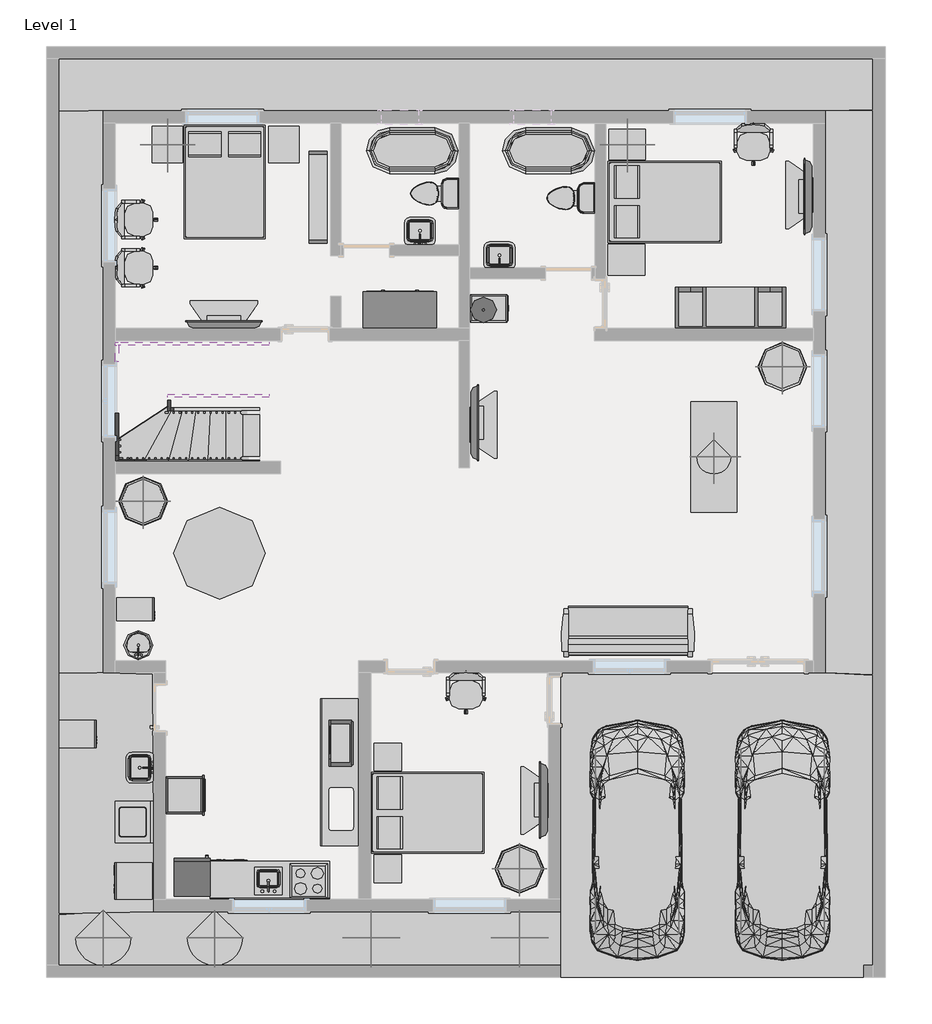
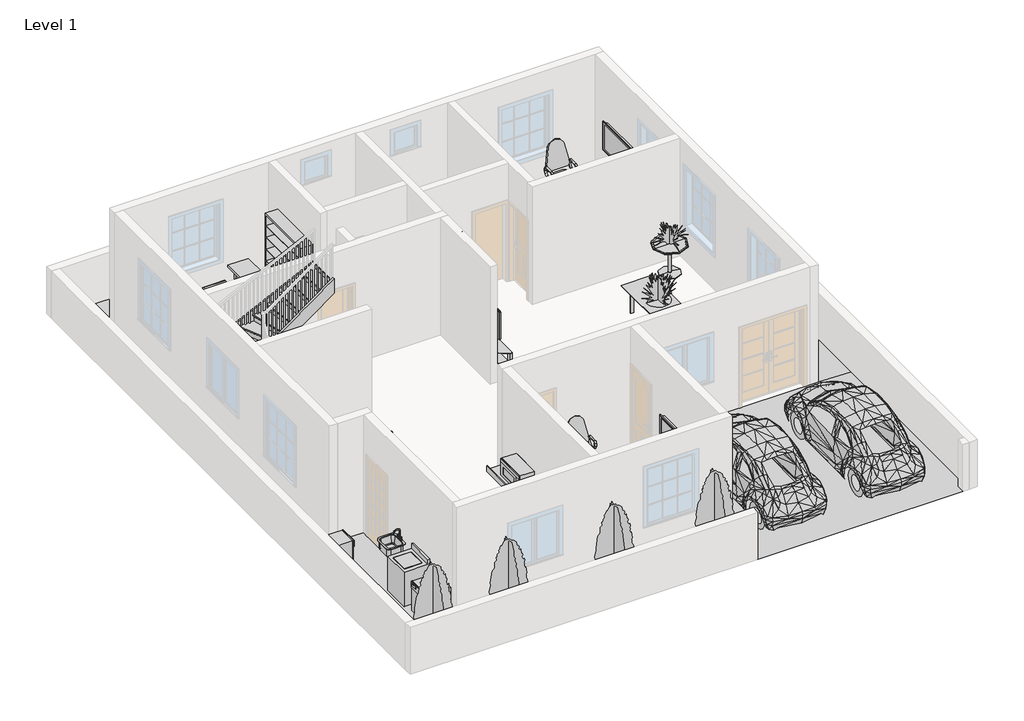
# One storey, part 3 of 3: 33 furniture elements, 18 proxies, 10 flow terminals, 10 geographic elements, 9 members, 1 stair flight.
"""IFC4 building model written with IfcOpenShell, lengths in millimetres."""

from ifc_helpers import new_model, si_unit, frame, origin, place, context, project, spatial, polyline, outline, extrude, triangles, transform, mapped, element, save
from components import proxy_db4bb64d, proxy_7e1014cc, proxy_a6faaae8, proxy_45b28599, kitchenette_medium_kitchenette_medium_844211aa, proxy_8a8d5ab2, proxy_f893816d, rpc_beetle_rpc_beetle_3ce7ba48, proxy_c523a7b7, proxy_718fa39f, flow_terminal_871c2e40, flow_terminal_d49f872f, flow_terminal_62a433f7, toilet_domestic_3d_toilet_domestic_3d_f7549cf7, toilet_domestic_3d_toilet_domestic_3d_183bbd19, flow_terminal_b374fae2, furniture_3e5ce493, furniture_c8abb964, chair_executive_chair_executive_8d69e98c, furniture_22cae41e, furniture_c6510c7c, furniture_9fa109b2, furniture_cf0b6580, furniture_b7bad97b, furniture_aff9b2fb, furniture_fdf74506, tv_stand_tv_stand_6ce107e5, furniture_c1c323c4, furniture_bbcc68ce, furniture_097b63cf, furniture_a4b90d56, furniture_eb3cba1b, rpc_plant_tropical_agave_1_5_93a2a214, rpc_plant_tropical_dagger_2_80c14bd7, rpc_tree_conifer_chinese_juniper_7_1b9786cd, stair_flight_2a3e21a6

model = new_model("IFC4")

# Units and contexts
model_context = context("Model", 3, world=origin())
ifc_project = project(units=[si_unit("LENGTHUNIT", "METRE", prefix="MILLI")], contexts=[model_context])

# Site, building, storey
site = spatial("IfcSite", under=ifc_project)
building = spatial("IfcBuilding", under=site)
storey = spatial("IfcBuildingStorey", under=building, Name="Level 1", Elevation=0.0)

# Proxies
placement = place(None, origin())
element("IfcBuildingElementProxy", 1, Name="Building Element Proxy", at=placement, inside=storey, context=model_context, shape_type="Tessellation", body=[
    triangles([(-7253.8729294, -205.6837934, 0.0), (-7253.8729294, 683.3162127, 0.0), (-15585.0731232, 631.8320005, 0.0), (-15585.0731232, -205.6837934, 0.0), (-14010.2727356, 729.26101, 0.0)], [[3, 4, 5], [5, 1, 2], [1, 5, 4]], closed=False),
])
element("IfcBuildingElementProxy", 2, Name="Building Element Proxy", at=placement, inside=storey, context=model_context, shape_type="Tessellation", body=[
    triangles([(-14848.4727356, 4645.71614, 0.0), (-15585.0731232, 4637.9227203, 0.0), (-14848.4727356, 13967.5160431, 0.0), (-15585.0731232, 13944.0349182, 0.0), (-15585.0731232, 13962.9767853, 0.0)], [[4, 3, 5], [4, 1, 3], [1, 4, 2]], closed=False),
])
element("IfcBuildingElementProxy", 3, Name="Building Element Proxy", at=placement, inside=storey, context=model_context, shape_type="Tessellation", body=[
    triangles([(-15585.0731232, 13966.5149414, 0.0), (-15585.0731232, 14831.1156555, 0.0), (-14848.4727356, 13967.5160431, 0.0), (-2859.6731232, 13967.5160431, 0.0), (-2072.2732201, 13984.9219574, 0.0), (-2072.2732201, 14831.1156555, 0.0)], [[2, 1, 3], [3, 1, 4], [2, 3, 4], [4, 5, 6], [4, 6, 2]], closed=False),
])
element("IfcBuildingElementProxy", 4, Name="Building Element Proxy", at=placement, inside=storey, context=model_context, shape_type="Tessellation", body=[
    triangles([(-2859.6731232, 13967.5160431, 0.0), (-2072.2732201, 13974.548172, 0.0), (-2859.6731232, 4645.71614, 0.0), (-2072.2732201, 4695.0738831, 0.0), (-2072.2732201, 4609.9508812, 0.0)], [[1, 3, 4], [4, 2, 1], [5, 4, 3]], closed=False),
])
element("IfcBuildingElementProxy", 5, Name="Building Element Proxy", at=placement, inside=storey, context=model_context, shape_type="Tessellation", body=[
    triangles([(-14033.0411133, 4622.8567795, 0.0), (-15585.0731232, 4585.4709801, 0.0), (-14010.2727356, 683.3162127, 0.0), (-15585.0731232, 648.3530851, 0.0), (-14848.4727356, 4645.71614, 0.0), (-15585.0731232, 4640.1260742, 0.0)], [[3, 5, 4], [2, 4, 5], [6, 2, 5], [5, 3, 1]], closed=False),
])
element("IfcBuildingElementProxy", 6, Name="Building Element Proxy", at=placement, inside=storey, context=model_context, shape_type="Tessellation", body=[
    triangles([(-7253.8729294, 4645.71614, 0.0), (-2859.6731232, 4645.71614, 0.0), (-2072.2732201, 4604.7651512, 0.0), (-2072.2732201, -205.6837934, 0.0), (-7253.8729294, -205.6837934, 0.0), (-7253.8729294, -408.8837995, 0.0), (-2224.6732201, -408.8837995, 0.0)], [[4, 5, 7], [5, 6, 7], [1, 5, 2], [4, 2, 5], [3, 2, 4]], closed=False),
])
proxy_shape = proxy_db4bb64d(model_context)
element("IfcBuildingElementProxy", 7, Name="15\" x 24\" x 34 1/2\"", ObjectType="15\" x 24\" x 34 1/2\"", at=placement, inside=storey, context=model_context, shape_type="MappedRepresentation", body=[
    mapped(proxy_shape, transform((-14048.6235886, 5431.7987427, 0.0), x_axis=(0.0, 1.0, 0.0), y_axis=(-1.0, 0.0, 0.0), z_axis=(0.0, 0.0, 1.0))),
])
proxy_2_shape = proxy_7e1014cc(model_context)
element("IfcBuildingElementProxy", 8, Name="18\" x 24\" x 34 1/2\"", ObjectType="18\" x 24\" x 34 1/2\"", at=placement, inside=storey, context=model_context, shape_type="MappedRepresentation", body=[
    mapped(proxy_2_shape, transform((-15013.8235886, 3323.5987427, 0.0), x_axis=(0.0, 1.0000000000000002, 0.0), y_axis=(-1.0000000000000002, 0.0, 0.0), z_axis=(0.0, 0.0, 1.0))),
])
proxy_3_shape = proxy_a6faaae8(model_context)
element("IfcBuildingElementProxy", 9, Name="Cook Top-4 Unit2 : 22\" x 20\"", ObjectType="Cook Top-4 Unit2 : 22\" x 20\"", at=placement, inside=storey, context=model_context, shape_type="MappedRepresentation", body=[
    mapped(proxy_3_shape, transform((-11432.1731534, 1191.3162111, 0.0), x_axis=(-1.0000000000000004, 0.0, 0.0), y_axis=(0.0, -1.0000000000000004, 0.0), z_axis=(0.0, 0.0, 1.0))),
])
proxy_4_shape = proxy_45b28599(model_context)
element("IfcBuildingElementProxy", 10, Name="Dishwasher : 24\" x 24\" x 34\"", ObjectType="Dishwasher : 24\" x 24\" x 34\"", at=placement, inside=storey, context=model_context, shape_type="MappedRepresentation", body=[
    mapped(proxy_4_shape, transform((-12383.3556849, 1483.1657759, 0.0), x_axis=(-1.0000000000000004, 0.0, 0.0), y_axis=(0.0, -1.0000000000000004, 0.0), z_axis=(0.0, 0.0, 1.0))),
])
element("IfcBuildingElementProxy", 11, Name="Dishwasher : 24\" x 24\" x 34\"", ObjectType="Dishwasher : 24\" x 24\" x 34\"", at=placement, inside=storey, context=model_context, shape_type="MappedRepresentation", body=[
    mapped(proxy_4_shape, transform((-14606.9227182, 1573.6336796, 0.0), x_axis=(0.0, -1.0000000000000002, 0.0), y_axis=(1.0000000000000002, 0.0, 0.0), z_axis=(0.0, 0.0, 1.0))),
])
kitchenette_medium_kitchenette_medium_shape = kitchenette_medium_kitchenette_medium_844211aa(model_context)
element("IfcBuildingElementProxy", 12, Name="Kitchenette - Medium : Kitchenette - Medium", ObjectType="Kitchenette - Medium : Kitchenette - Medium", at=placement, inside=storey, context=model_context, shape_type="MappedRepresentation", body=[
    mapped(kitchenette_medium_kitchenette_medium_shape, transform((-11756.3354485, 886.5162111, 0.0), x_axis=(-1.0000000000000004, 0.0, 0.0), y_axis=(0.0, -1.0000000000000004, 0.0), z_axis=(0.0, 0.0, 1.0))),
])
proxy_5_shape = proxy_8a8d5ab2(model_context)
element("IfcBuildingElementProxy", 13, Name="Microwave : 30\" x 16\" x 18\"", ObjectType="Microwave : 30\" x 16\" x 18\"", at=placement, inside=storey, context=model_context, shape_type="MappedRepresentation", body=[
    mapped(proxy_5_shape, transform((-10545.6926476, 3977.6090885, 0.0), x_axis=(0.0, -1.0000000000000004, 0.0), y_axis=(1.0000000000000004, 0.0, 0.0), z_axis=(0.0, 0.0, 1.0))),
])
proxy_6_shape = proxy_f893816d(model_context)
element("IfcBuildingElementProxy", 14, Name="Oven Double-Built-in : 24 1/4\" x 50 3/8\" x 24\"", ObjectType="Oven Double-Built-in : 24 1/4\" x 50 3/8\" x 24\"", at=placement, inside=storey, context=model_context, shape_type="MappedRepresentation", body=[
    mapped(proxy_6_shape, transform((-13361.2072944, 2648.8911385, 0.0), x_axis=(0.0, 1.0000000000000002, 0.0), y_axis=(-1.0000000000000002, 0.0, 0.0), z_axis=(0.0, 0.0, 1.0))),
])
rpc_beetle_rpc_beetle_shape = rpc_beetle_rpc_beetle_3ce7ba48(model_context)
element("IfcBuildingElementProxy", 15, Name="RPC Beetle : RPC Beetle", ObjectType="RPC Beetle : RPC Beetle", at=placement, inside=storey, context=model_context, shape_type="MappedRepresentation", body=[
    mapped(rpc_beetle_rpc_beetle_shape, transform((-5983.8731534, 632.5162111, 0.0), x_axis=(1.0, 0.0, 0.0), y_axis=(0.0, 1.0, 0.0), z_axis=(0.0, 0.0, 1.0))),
])
element("IfcBuildingElementProxy", 16, Name="RPC Beetle : RPC Beetle", ObjectType="RPC Beetle : RPC Beetle", at=placement, inside=storey, context=model_context, shape_type="MappedRepresentation", body=[
    mapped(rpc_beetle_rpc_beetle_shape, transform((-3570.8731534, 632.5162111, 0.0), x_axis=(1.0, 0.0, 0.0), y_axis=(0.0, 1.0, 0.0), z_axis=(0.0, 0.0, 1.0))),
])
proxy_7_shape = proxy_c523a7b7(model_context)
element("IfcBuildingElementProxy", 17, Name="Refrigerator : 24\" x 25\" LH", ObjectType="Refrigerator : 24\" x 25\" LH", at=placement, inside=storey, context=model_context, shape_type="MappedRepresentation", body=[
    mapped(proxy_7_shape, transform((-13368.9231534, 1236.9651826, 0.0), x_axis=(-1.0000000000000004, 0.0, 0.0), y_axis=(0.0, -1.0000000000000004, 0.0), z_axis=(0.0, 0.0, 1.0))),
])
proxy_8_shape = proxy_718fa39f(model_context)
element("IfcBuildingElementProxy", 18, Name="Washer : 27\" x 25\" x 35\"", ObjectType="Washer : 27\" x 25\" x 35\"", at=placement, inside=storey, context=model_context, shape_type="MappedRepresentation", body=[
    mapped(proxy_8_shape, transform((-14606.9227182, 2589.6336796, 0.0), x_axis=(0.0, -1.0000000000000002, 0.0), y_axis=(1.0000000000000002, 0.0, 0.0), z_axis=(0.0, 0.0, 1.0))),
])

# Flow terminals
flow_terminal_shape = flow_terminal_871c2e40(model_context)
element("IfcFlowTerminal", 19, ObjectType="Sink Kitchen-Island : 18\" x 18\"", at=placement, inside=storey, context=model_context, shape_type="MappedRepresentation", body=[
    mapped(flow_terminal_shape, transform((-12089.5839128, 1193.6616123, -14.4), x_axis=(-1.0000000000000004, 0.0, 0.0), y_axis=(0.0, -1.0000000000000004, 0.0), z_axis=(0.0, 0.0, 1.0))),
])
flow_terminal_2_shape = flow_terminal_d49f872f(model_context)
element("IfcFlowTerminal", 20, ObjectType="Sink Vanity-Round : 19\" x 19\"", at=placement, inside=storey, context=model_context, shape_type="MappedRepresentation", body=[
    mapped(flow_terminal_2_shape, transform((-8450.5818516, 10568.8644706, 609.6), x_axis=(0.0, 1.0000000000000002, 0.0), y_axis=(-1.0000000000000002, 0.0, 0.0), z_axis=(0.0, 0.0, 1.0))),
])
element("IfcFlowTerminal", 21, ObjectType="Sink Vanity-Round : 19\" x 19\"", at=placement, inside=storey, context=model_context, shape_type="MappedRepresentation", body=[
    mapped(flow_terminal_2_shape, transform((-14167.6214128, 5187.9844901, 0.0), x_axis=(-1.0000000000000004, 0.0, 0.0), y_axis=(0.0, -1.0000000000000004, 0.0), z_axis=(0.0, 0.0, 1.0))),
])
flow_terminal_3_shape = flow_terminal_62a433f7(model_context)
element("IfcFlowTerminal", 22, ObjectType="Sink Vanity-Square : 20\" x 18\"", at=placement, inside=storey, context=model_context, shape_type="MappedRepresentation", body=[
    mapped(flow_terminal_3_shape, transform((-9574.9839128, 11925.1616123, 0.0), x_axis=(-1.0, 0.0, 0.0), y_axis=(0.0, -1.0, 0.0), z_axis=(0.0, 0.0, 1.0))),
])
element("IfcFlowTerminal", 23, ObjectType="Sink Vanity-Square : 20\" x 18\"", at=placement, inside=storey, context=model_context, shape_type="MappedRepresentation", body=[
    mapped(flow_terminal_3_shape, transform((-8254.1839128, 11518.7616123, 0.0), x_axis=(-1.0, 0.0, 0.0), y_axis=(0.0, -1.0, 0.0), z_axis=(0.0, 0.0, 1.0))),
])
element("IfcFlowTerminal", 24, ObjectType="Sink Vanity-Square : 20\" x 18\"", at=placement, inside=storey, context=model_context, shape_type="MappedRepresentation", body=[
    mapped(flow_terminal_3_shape, transform((-14190.4185545, 3086.6054517, 0.0), x_axis=(0.0, -1.0000000000000002, 0.0), y_axis=(1.0000000000000002, 0.0, 0.0), z_axis=(0.0, 0.0, 1.0))),
])
toilet_domestic_3d_toilet_domestic_3d_shape = toilet_domestic_3d_toilet_domestic_3d_f7549cf7(model_context)
toilet_domestic_3d_toilet_domestic_3d_2_shape = toilet_domestic_3d_toilet_domestic_3d_183bbd19(model_context)
element("IfcFlowTerminal", 25, ObjectType="Toilet-Domestic-3D : Toilet-Domestic-3D", at=placement, inside=storey, context=model_context, shape_type="MappedRepresentation", body=[
    mapped(toilet_domestic_3d_toilet_domestic_3d_shape, transform((-9437.6691807, 12595.9162111, 0.0), x_axis=(0.0, -1.0000000000000004, 0.0), y_axis=(1.0000000000000004, 0.0, 0.0), z_axis=(0.0, 0.0, 1.0))),
    mapped(toilet_domestic_3d_toilet_domestic_3d_2_shape, transform((-9437.6691807, 12595.9162111, 0.0), x_axis=(0.0, -1.0000000000000004, 0.0), y_axis=(1.0000000000000004, 0.0, 0.0), z_axis=(0.0, 0.0, 1.0))),
])
element("IfcFlowTerminal", 26, ObjectType="Toilet-Domestic-3D : Toilet-Domestic-3D", at=placement, inside=storey, context=model_context, shape_type="MappedRepresentation", body=[
    mapped(toilet_domestic_3d_toilet_domestic_3d_shape, transform((-7177.0691807, 12519.7162111, 0.0), x_axis=(0.0, -1.0, 0.0), y_axis=(1.0, 0.0, 0.0), z_axis=(0.0, 0.0, 1.0))),
    mapped(toilet_domestic_3d_toilet_domestic_3d_2_shape, transform((-7177.0691807, 12519.7162111, 0.0), x_axis=(0.0, -1.0, 0.0), y_axis=(1.0, 0.0, 0.0), z_axis=(0.0, 0.0, 1.0))),
])
flow_terminal_4_shape = flow_terminal_b374fae2(model_context)
element("IfcFlowTerminal", 27, ObjectType="Tub-Free Standing-3D : 30\" x 60\"", at=placement, inside=storey, context=model_context, shape_type="MappedRepresentation", body=[
    mapped(flow_terminal_4_shape, transform((-7457.0731534, 13307.1162111, 0.0), x_axis=(0.0, -1.0, 0.0), y_axis=(1.0, 0.0, 0.0), z_axis=(0.0, 0.0, 1.0))),
])
element("IfcFlowTerminal", 28, ObjectType="Tub-Free Standing-3D : 30\" x 60\"", at=placement, inside=storey, context=model_context, shape_type="MappedRepresentation", body=[
    mapped(flow_terminal_4_shape, transform((-9717.6731534, 13307.1162111, 0.0), x_axis=(0.0, -1.0, 0.0), y_axis=(1.0, 0.0, 0.0), z_axis=(0.0, 0.0, 1.0))),
])

# Furniture
furniture_shape = furniture_3e5ce493(model_context)
element("IfcFurniture", 29, ObjectType="Base Cabinet-2 Bin : 18\"", at=placement, inside=storey, context=model_context, shape_type="MappedRepresentation", body=[
    mapped(furniture_shape, transform((-8751.6495701, 10672.1785062, 0.0), x_axis=(0.0, 1.0000000000000002, 0.0), y_axis=(-1.0000000000000002, 0.0, 0.0), z_axis=(0.0, 0.0, 1.0))),
])
furniture_2_shape = furniture_c8abb964(model_context)
element("IfcFurniture", 30, ObjectType="Bed-Box : Double 53\" x 74\"", at=placement, inside=storey, context=model_context, shape_type="MappedRepresentation", body=[
    mapped(furniture_2_shape, transform((-13168.3256124, 13020.8457193, 0.0), x_axis=(1.0, 0.0, 0.0), y_axis=(0.0, 1.0, 0.0), z_axis=(0.0, 0.0, 1.0))),
])
element("IfcFurniture", 31, ObjectType="Bed-Box : Double 53\" x 74\"", at=placement, inside=storey, context=model_context, shape_type="MappedRepresentation", body=[
    mapped(furniture_2_shape, transform((-5761.1026616, 12117.0637521, 0.0), x_axis=(0.0, 1.0, 0.0), y_axis=(-1.0, 0.0, 0.0), z_axis=(0.0, 0.0, 1.0))),
])
element("IfcFurniture", 32, ObjectType="Bed-Box : Double 53\" x 74\"", at=placement, inside=storey, context=model_context, shape_type="MappedRepresentation", body=[
    mapped(furniture_2_shape, transform((-9698.1026616, 1982.4637521, 0.0), x_axis=(0.0, 1.0, 0.0), y_axis=(-1.0, 0.0, 0.0), z_axis=(0.0, 0.0, 1.0))),
])
chair_executive_chair_executive_shape = chair_executive_chair_executive_8d69e98c(model_context)
element("IfcFurniture", 33, ObjectType="Chair-Executive : Chair-Executive", at=placement, inside=storey, context=model_context, shape_type="MappedRepresentation", body=[
    mapped(chair_executive_chair_executive_shape, transform((-14308.619055, 12305.1070308, 0.0), x_axis=(0.0, -1.0000000000000004, 0.0), y_axis=(1.0000000000000004, 0.0, 0.0), z_axis=(0.0, 0.0, 1.0))),
])
element("IfcFurniture", 34, ObjectType="Chair-Executive : Chair-Executive", at=placement, inside=storey, context=model_context, shape_type="MappedRepresentation", body=[
    mapped(chair_executive_chair_executive_shape, transform((-14308.619055, 11505.0070308, 0.0), x_axis=(0.0, -1.0, 0.0), y_axis=(1.0, 0.0, 0.0), z_axis=(0.0, 0.0, 1.0))),
])
element("IfcFurniture", 35, ObjectType="Chair-Executive : Chair-Executive", at=placement, inside=storey, context=model_context, shape_type="MappedRepresentation", body=[
    mapped(chair_executive_chair_executive_shape, transform((-3912.4823337, 13427.6621128, 0.0), x_axis=(-1.0000000000000004, 0.0, 0.0), y_axis=(0.0, -1.0000000000000004, 0.0), z_axis=(0.0, 0.0, 1.0))),
])
element("IfcFurniture", 36, ObjectType="Chair-Executive : Chair-Executive", at=placement, inside=storey, context=model_context, shape_type="MappedRepresentation", body=[
    mapped(chair_executive_chair_executive_shape, transform((-8687.6823337, 4334.4621128, 0.0), x_axis=(-1.0000000000000004, 0.0, 0.0), y_axis=(0.0, -1.0000000000000004, 0.0), z_axis=(0.0, 0.0, 1.0))),
])
furniture_3_shape = furniture_22cae41e(model_context)
element("IfcFurniture", 37, ObjectType="Counter Top w Sink Hole : 24\" Depth", at=placement, inside=storey, context=model_context, shape_type="MappedRepresentation", body=[
    mapped(furniture_3_shape, transform((-11241.6731534, 2975.9785062, 0.0), x_axis=(0.0, 1.0000000000000002, 0.0), y_axis=(-1.0000000000000002, 0.0, 0.0), z_axis=(0.0, 0.0, 1.0))),
])
furniture_4_shape = furniture_c6510c7c(model_context)
element("IfcFurniture", 38, ObjectType="Counter Top w Sink Hole : 24\" Depth", at=placement, inside=storey, context=model_context, shape_type="MappedRepresentation", body=[
    mapped(furniture_4_shape, transform((-12289.7354485, 886.5162111, -14.4), x_axis=(-1.0000000000000004, 0.0, 0.0), y_axis=(0.0, -1.0000000000000004, 0.0), z_axis=(0.0, 0.0, 1.0))),
])
furniture_5_shape = furniture_9fa109b2(model_context)
element("IfcFurniture", 39, ObjectType="Dresser : 48\" x 72\" x 24\"", at=placement, inside=storey, context=model_context, shape_type="MappedRepresentation", body=[
    mapped(furniture_5_shape, transform((-10190.0664132, 10302.3532571, 0.0), x_axis=(-1.0000000000000007, 0.0, 0.0), y_axis=(0.0, -1.0000000000000007, 0.0), z_axis=(0.0, 0.0, 1.0))),
])
furniture_6_shape = furniture_cf0b6580(model_context)
element("IfcFurniture", 40, ObjectType="Entertainment Center : 72\" x 72\" x 24\"", at=placement, inside=storey, context=model_context, shape_type="MappedRepresentation", body=[
    mapped(furniture_6_shape, transform((-4434.4731534, 10259.1162111, 0.0), x_axis=(-1.0000000000000004, 0.0, 0.0), y_axis=(0.0, -1.0000000000000004, 0.0), z_axis=(0.0, 0.0, 1.0))),
])
furniture_7_shape = furniture_b7bad97b(model_context)
element("IfcFurniture", 41, ObjectType="Shelving : 96\" x 12\" x 84\"", at=placement, inside=storey, context=model_context, shape_type="MappedRepresentation", body=[
    mapped(furniture_7_shape, transform((-11584.5731534, 12532.4162111, 0.0), x_axis=(0.0, 1.0000000000000002, 0.0), y_axis=(-1.0000000000000002, 0.0, 0.0), z_axis=(0.0, 0.0, 1.0))),
])
furniture_8_shape = furniture_aff9b2fb(model_context)
element("IfcFurniture", 42, ObjectType="Sofa-Pensi : 84\"", at=placement, inside=storey, context=model_context, shape_type="MappedRepresentation", body=[
    mapped(furniture_8_shape, transform((-5857.6669034, 5608.6260472, 0.0), x_axis=(-1.0000000000000004, 0.0, 0.0), y_axis=(0.0, -1.0000000000000004, 0.0), z_axis=(0.0, 0.0, 1.0))),
])
furniture_9_shape = furniture_fdf74506(model_context)
element("IfcFurniture", 43, ObjectType="TV - Flat Screen : 50\"", at=placement, inside=storey, context=model_context, shape_type="MappedRepresentation", body=[
    mapped(furniture_9_shape, transform((-12845.8176675, 10419.2548348, 914.4), x_axis=(-1.0000000000000007, 0.0, 0.0), y_axis=(0.0, -1.0000000000000007, 0.0), z_axis=(0.0, 0.0, 1.0))),
])
element("IfcFurniture", 44, ObjectType="TV - Flat Screen : 50\"", at=placement, inside=storey, context=model_context, shape_type="MappedRepresentation", body=[
    mapped(furniture_9_shape, transform((-3146.811777, 12541.171697, 914.4), x_axis=(0.0, -1.0, 0.0), y_axis=(1.0, 0.0, 0.0), z_axis=(0.0, 0.0, 1.0))),
])
element("IfcFurniture", 45, ObjectType="TV - Flat Screen : 50\"", at=placement, inside=storey, context=model_context, shape_type="MappedRepresentation", body=[
    mapped(furniture_9_shape, transform((-7535.611777, 2527.9537767, 914.4), x_axis=(0.0, -1.0, 0.0), y_axis=(1.0, 0.0, 0.0), z_axis=(0.0, 0.0, 1.0))),
])
element("IfcFurniture", 46, ObjectType="TV - Flat Screen : 50\"", at=placement, inside=storey, context=model_context, shape_type="MappedRepresentation", body=[
    mapped(furniture_9_shape, transform((-8686.6345297, 8796.9607253, 914.4), x_axis=(0.0, 1.0, 0.0), y_axis=(-1.0, 0.0, 0.0), z_axis=(0.0, 0.0, 1.0))),
])
tv_stand_tv_stand_shape = tv_stand_tv_stand_6ce107e5(model_context)
element("IfcFurniture", 47, ObjectType="TV Stand : TV Stand", at=placement, inside=storey, context=model_context, shape_type="MappedRepresentation", body=[
    mapped(tv_stand_tv_stand_shape, transform((-12716.6851513, 10360.7162111, 0.0), x_axis=(-1.0000000000000016, 0.0, 0.0), y_axis=(0.0, -1.0000000000000016, 0.0), z_axis=(0.0, 0.0, 1.0))),
])
element("IfcFurniture", 48, ObjectType="TV Stand : TV Stand", at=placement, inside=storey, context=model_context, shape_type="MappedRepresentation", body=[
    mapped(tv_stand_tv_stand_shape, transform((-3062.8731534, 12695.7042132, 0.0), x_axis=(0.0, -1.0, 0.0), y_axis=(1.0, 0.0, 0.0), z_axis=(0.0, 0.0, 1.0))),
])
element("IfcFurniture", 49, ObjectType="TV Stand : TV Stand", at=placement, inside=storey, context=model_context, shape_type="MappedRepresentation", body=[
    mapped(tv_stand_tv_stand_shape, transform((-7457.0731534, 2650.0042132, 0.0), x_axis=(0.0, -1.0, 0.0), y_axis=(1.0, 0.0, 0.0), z_axis=(0.0, 0.0, 1.0))),
])
element("IfcFurniture", 50, ObjectType="TV Stand : TV Stand", at=placement, inside=storey, context=model_context, shape_type="MappedRepresentation", body=[
    mapped(tv_stand_tv_stand_shape, transform((-8765.1731534, 8635.3282091, 0.0), x_axis=(0.0, 1.0000000000000002, 0.0), y_axis=(-1.0000000000000002, 0.0, 0.0), z_axis=(0.0, 0.0, 1.0))),
])
furniture_10_shape = furniture_c1c323c4(model_context)
element("IfcFurniture", 51, ObjectType="Table-Dining : 30\" x 84\" x 22\"", at=placement, inside=storey, context=model_context, shape_type="MappedRepresentation", body=[
    mapped(furniture_10_shape, transform((-4618.6620756, 8208.8504445, 0.0), x_axis=(0.0, 1.0000000000000002, 0.0), y_axis=(-1.0000000000000002, 0.0, 0.0), z_axis=(0.0, 0.0, 1.0))),
])
furniture_11_shape = furniture_bbcc68ce(model_context)
element("IfcFurniture", 52, ObjectType="Table-Dining Round w Chairs : 60\" Diameter", at=placement, inside=storey, context=model_context, shape_type="MappedRepresentation", body=[
    mapped(furniture_11_shape, transform((-13021.7551206, 6811.7948997, 0.0), x_axis=(1.0, 0.0, 0.0), y_axis=(0.0, 1.0, 0.0), z_axis=(0.0, 0.0, 1.0))),
])
furniture_12_shape = furniture_097b63cf(model_context)
element("IfcFurniture", 53, ObjectType="Table-Night Stand : 18\" x 18\" x 24\"", at=placement, inside=storey, context=model_context, shape_type="MappedRepresentation", body=[
    mapped(furniture_12_shape, transform((-10356.4067837, 1165.9162111, 0.0), x_axis=(1.0, 0.0, 0.0), y_axis=(0.0, 1.0, 0.0), z_axis=(0.0, 0.0, 1.0))),
])
element("IfcFurniture", 54, ObjectType="Table-Night Stand : 18\" x 18\" x 24\"", at=placement, inside=storey, context=model_context, shape_type="MappedRepresentation", body=[
    mapped(furniture_12_shape, transform((-10356.4067837, 3020.1162111, 0.0), x_axis=(1.0, 0.0, 0.0), y_axis=(0.0, 1.0, 0.0), z_axis=(0.0, 0.0, 1.0))),
])
furniture_13_shape = furniture_a4b90d56(model_context)
element("IfcFurniture", 55, ObjectType="Table-Night Stand : 24\" x 24\" x 30\"", at=placement, inside=storey, context=model_context, shape_type="MappedRepresentation", body=[
    mapped(furniture_13_shape, transform((-14039.4067837, 13103.9162111, 0.0), x_axis=(1.0, 0.0, 0.0), y_axis=(0.0, 1.0, 0.0), z_axis=(0.0, 0.0, 1.0))),
])
element("IfcFurniture", 56, ObjectType="Table-Night Stand : 24\" x 24\" x 30\"", at=placement, inside=storey, context=model_context, shape_type="MappedRepresentation", body=[
    mapped(furniture_13_shape, transform((-12109.0067837, 13103.9162111, 0.0), x_axis=(1.0, 0.0, 0.0), y_axis=(0.0, 1.0, 0.0), z_axis=(0.0, 0.0, 1.0))),
])
element("IfcFurniture", 57, ObjectType="Table-Night Stand : 24\" x 24\" x 30\"", at=placement, inside=storey, context=model_context, shape_type="MappedRepresentation", body=[
    mapped(furniture_13_shape, transform((-5844.1731534, 13150.9825809, 0.0), x_axis=(0.0, 1.0000000000000002, 0.0), y_axis=(-1.0000000000000002, 0.0, 0.0), z_axis=(0.0, 0.0, 1.0))),
])
element("IfcFurniture", 58, ObjectType="Table-Night Stand : 24\" x 24\" x 30\"", at=placement, inside=storey, context=model_context, shape_type="MappedRepresentation", body=[
    mapped(furniture_13_shape, transform((-5856.8731534, 11239.6325809, 0.0), x_axis=(0.0, 1.0000000000000002, 0.0), y_axis=(-1.0000000000000002, 0.0, 0.0), z_axis=(0.0, 0.0, 1.0))),
])
furniture_14_shape = furniture_eb3cba1b(model_context)
element("IfcFurniture", 59, ObjectType="Table-Round : 36\" Diameter", at=placement, inside=storey, context=model_context, shape_type="MappedRepresentation", body=[
    mapped(furniture_14_shape, transform((-7939.6731534, 1394.5162111, 0.0), x_axis=(1.0, 0.0, 0.0), y_axis=(0.0, 1.0, 0.0), z_axis=(0.0, 0.0, 1.0))),
])
element("IfcFurniture", 60, ObjectType="Table-Round : 36\" Diameter", at=placement, inside=storey, context=model_context, shape_type="MappedRepresentation", body=[
    mapped(furniture_14_shape, transform((-14184.3414615, 7490.5162111, 0.0), x_axis=(1.0, 0.0, 0.0), y_axis=(0.0, 1.0, 0.0), z_axis=(0.0, 0.0, 1.0))),
])
element("IfcFurniture", 61, ObjectType="Table-Round : 36\" Diameter", at=placement, inside=storey, context=model_context, shape_type="MappedRepresentation", body=[
    mapped(furniture_14_shape, transform((-3570.8731534, 9719.3662111, 0.0), x_axis=(1.0, 0.0, 0.0), y_axis=(0.0, 1.0, 0.0), z_axis=(0.0, 0.0, 1.0))),
])

# Geographic elements
rpc_plant_tropical_agave_1_5_shape = rpc_plant_tropical_agave_1_5_93a2a214(model_context)
element("IfcGeographicElement", 62, ObjectType="RPC Plant - Tropical : Agave - 1.5'", at=placement, inside=storey, context=model_context, shape_type="MappedRepresentation", body=[
    mapped(rpc_plant_tropical_agave_1_5_shape, transform((-3570.8731534, 9719.3662111, 762.0), x_axis=(1.0, 0.0, 0.0), y_axis=(0.0, 1.0, 0.0), z_axis=(0.0, 0.0, 1.0))),
])
element("IfcGeographicElement", 63, ObjectType="RPC Plant - Tropical : Agave - 1.5'", at=placement, inside=storey, context=model_context, shape_type="MappedRepresentation", body=[
    mapped(rpc_plant_tropical_agave_1_5_shape, transform((-14184.3414615, 7490.5162111, 762.0), x_axis=(1.0, 0.0, 0.0), y_axis=(0.0, 1.0, 0.0), z_axis=(0.0, 0.0, 1.0))),
])
element("IfcGeographicElement", 64, ObjectType="RPC Plant - Tropical : Agave - 1.5'", at=placement, inside=storey, context=model_context, shape_type="MappedRepresentation", body=[
    mapped(rpc_plant_tropical_agave_1_5_shape, transform((-13781.6731534, 13408.7162111, 762.0), x_axis=(1.0, 0.0, 0.0), y_axis=(0.0, 1.0, 0.0), z_axis=(0.0, 0.0, 1.0))),
])
element("IfcGeographicElement", 65, ObjectType="RPC Plant - Tropical : Agave - 1.5'", at=placement, inside=storey, context=model_context, shape_type="MappedRepresentation", body=[
    mapped(rpc_plant_tropical_agave_1_5_shape, transform((-7939.6731534, 1394.5162111, 0.0), x_axis=(1.0, 0.0, 0.0), y_axis=(0.0, 1.0, 0.0), z_axis=(0.0, 0.0, 1.0))),
])
element("IfcGeographicElement", 66, ObjectType="RPC Plant - Tropical : Agave - 1.5'", at=placement, inside=storey, context=model_context, shape_type="MappedRepresentation", body=[
    mapped(rpc_plant_tropical_agave_1_5_shape, transform((-6148.9731534, 13408.7162111, 762.0), x_axis=(1.0, 0.0, 0.0), y_axis=(0.0, 1.0, 0.0), z_axis=(0.0, 0.0, 1.0))),
])
rpc_plant_tropical_dagger_2_shape = rpc_plant_tropical_dagger_2_80c14bd7(model_context)
element("IfcGeographicElement", 67, ObjectType="RPC Plant - Tropical : Dagger - 2'", at=placement, inside=storey, context=model_context, shape_type="MappedRepresentation", body=[
    mapped(rpc_plant_tropical_dagger_2_shape, transform((-4713.8731534, 8227.1162111, 609.6), x_axis=(1.0, 0.0, 0.0), y_axis=(0.0, 1.0, 0.0), z_axis=(0.0, 0.0, 1.0))),
])
rpc_tree_conifer_chinese_juniper_7_shape = rpc_tree_conifer_chinese_juniper_7_1b9786cd(model_context)
element("IfcGeographicElement", 68, ObjectType="RPC Tree - Conifer : Chinese Juniper - 7'", at=placement, inside=storey, context=model_context, shape_type="MappedRepresentation", body=[
    mapped(rpc_tree_conifer_chinese_juniper_7_shape, transform((-7939.8698245, 251.5162111, 0.0), x_axis=(1.0, 0.0, 0.0), y_axis=(0.0, 1.0, 0.0), z_axis=(0.0, 0.0, 1.0))),
])
element("IfcGeographicElement", 69, ObjectType="RPC Tree - Conifer : Chinese Juniper - 7'", at=placement, inside=storey, context=model_context, shape_type="MappedRepresentation", body=[
    mapped(rpc_tree_conifer_chinese_juniper_7_shape, transform((-10403.6698245, 251.5162111, 0.0), x_axis=(1.0, 0.0, 0.0), y_axis=(0.0, 1.0, 0.0), z_axis=(0.0, 0.0, 1.0))),
])
element("IfcGeographicElement", 70, ObjectType="RPC Tree - Conifer : Chinese Juniper - 7'", at=placement, inside=storey, context=model_context, shape_type="MappedRepresentation", body=[
    mapped(rpc_tree_conifer_chinese_juniper_7_shape, transform((-12994.4698245, 251.5162111, 0.0), x_axis=(1.0, 0.0, 0.0), y_axis=(0.0, 1.0, 0.0), z_axis=(0.0, 0.0, 1.0))),
])
element("IfcGeographicElement", 71, ObjectType="RPC Tree - Conifer : Chinese Juniper - 7'", at=placement, inside=storey, context=model_context, shape_type="MappedRepresentation", body=[
    mapped(rpc_tree_conifer_chinese_juniper_7_shape, transform((-14848.6698245, 251.5162111, 0.0), x_axis=(1.0, 0.0, 0.0), y_axis=(0.0, 1.0, 0.0), z_axis=(0.0, 0.0, 1.0))),
])

# Members
element("IfcMember", 72, ObjectType="Stringer - 2\" Width", at=placement, inside=storey, context=model_context, shape_type="SweptSolid", body=[
    extrude(outline(polyline([(0.0, -12253.9414615), (229.0091112, -12253.9414615), (1305.2117081, -14329.5439617), (961.875972, -14329.5439617), (0.0, -12474.4358453), (0.0, -12253.9414615)])), frame((0.0, 8125.5162111, 0.0), z_axis=(0.0, 1.0, 0.0), x_axis=(0.0, 0.0, 1.0)), (0.0, 0.0, 1.0), 50.8),
])
element("IfcMember", 73, ObjectType="Stringer - 2\" Width", at=placement, inside=storey, context=model_context, shape_type="SweptSolid", body=[
    extrude(outline(polyline([(-14329.5439617, 8176.3162111), (-14329.5439617, 8125.5162111), (-14645.2731534, 8125.5162111), (-14594.4731534, 8176.3162111), (-14329.5439617, 8176.3162111)])), frame((0.0, 0.0, 961.875972), z_axis=(0.0, 0.0, 1.0), x_axis=(1.0, 0.0, 0.0)), (0.0, 0.0, 1.0), 343.3357361),
])
element("IfcMember", 74, ObjectType="Stringer - 2\" Width", at=placement, inside=storey, context=model_context, shape_type="SweptSolid", body=[
    extrude(outline(polyline([(-14594.4731534, 8176.3162111), (-14645.2731534, 8125.5162111), (-14645.2731534, 8243.3346294), (-14594.4731534, 8243.3346294), (-14594.4731534, 8176.3162111)])), frame((0.0, 0.0, 961.875972), z_axis=(0.0, 0.0, 1.0), x_axis=(1.0, 0.0, 0.0)), (0.0, 0.0, 1.0), 343.3357361),
])
element("IfcMember", 75, ObjectType="Stringer - 2\" Width", at=placement, inside=storey, context=model_context, shape_type="SweptSolid", body=[
    extrude(outline(polyline([(8243.3346294, 961.875972), (8243.3346294, 1305.2117081), (9802.9632453, 1828.1543528), (9802.9632453, 1484.8186167), (8243.3346294, 961.875972)])), frame((-14645.2731534, 0.0, 0.0), z_axis=(1.0, 0.0, 0.0), x_axis=(0.0, 1.0, 0.0)), (0.0, 0.0, 1.0), 50.8),
])
element("IfcMember", 76, ObjectType="Stringer - 2\" Width", at=placement, inside=storey, context=model_context, shape_type="SweptSolid", body=[
    extrude(outline(polyline([(-14594.4731534, 9802.9632453), (-14645.2731534, 9802.9632453), (-14645.2731534, 10081.3162111), (-14594.4731534, 10081.3162111), (-14594.4731534, 9802.9632453)])), frame((0.0, 0.0, 1495.1890905), z_axis=(0.0, 0.0, 1.0), x_axis=(1.0, 0.0, 0.0)), (0.0, 0.0, 1.0), 321.4774213),
])
element("IfcMember", 77, ObjectType="Stringer - 2\" Width", at=placement, inside=storey, context=model_context, shape_type="SweptSolid", body=[
    extrude(outline(polyline([(0.0, -12253.9414615), (193.149682, -12253.9414615), (1245.2345891, -13730.8731534), (871.0082789, -13730.8731534), (0.0, -12508.1393966), (0.0, -12253.9414615)])), frame((0.0, 8989.1162111, 0.0), z_axis=(0.0, 1.0, 0.0), x_axis=(0.0, 0.0, 1.0)), (0.0, 0.0, 1.0), 50.8),
])
element("IfcMember", 78, ObjectType="Stringer - 2\" Width", at=placement, inside=storey, context=model_context, shape_type="SweptSolid", body=[
    extrude(outline(polyline([(8989.1162111, 907.1954049), (8989.1162111, 1530.0908825), (9176.7922221, 1905.1630186), (9217.7162111, 1905.1630186), (9217.7162111, 1305.8029828), (9018.263698, 907.1954049), (8989.1162111, 907.1954049)])), frame((-13781.6731534, 0.0, 0.0), z_axis=(1.0, 0.0, 0.0), x_axis=(0.0, 1.0, 0.0)), (0.0, 0.0, 1.0), 50.8),
])
element("IfcMember", 79, ObjectType="Stringer - 2\" Width", at=placement, inside=storey, context=model_context, shape_type="SweptSolid", body=[
    extrude(outline(polyline([(1905.1630186, -13781.6731534), (1527.8638327, -13781.6731534), (2760.6108416, -12092.016007), (3137.9100276, -12092.016007), (1905.1630186, -13781.6731534)])), frame((0.0, 9217.7162111, 0.0), z_axis=(0.0, 1.0, 0.0), x_axis=(0.0, 0.0, 1.0)), (0.0, 0.0, 1.0), 50.8),
])
element("IfcMember", 80, ObjectType="Stringer - 2\" Width", at=placement, inside=storey, context=model_context, shape_type="SweptSolid", body=[
    extrude(outline(polyline([(1791.8561823, -14645.2731534), (1511.8665118, -14645.2731534), (1511.8665118, -14560.3255618), (2717.3699248, -12092.016007), (3038.847346, -12092.016007), (1791.8561823, -14645.2731534)])), frame((0.0, 10081.3162111, 0.0), z_axis=(0.0, 1.0, 0.0), x_axis=(0.0, 0.0, 1.0)), (0.0, 0.0, 1.0), 50.8),
])

# Stair flight
stair_flight_shape = stair_flight_2a3e21a6(model_context)
element("IfcStairFlight", 81, ObjectType="2\" Tread 1\" Nosing 1/4\" Riser", at=placement, inside=storey, context=model_context, shape_type="MappedRepresentation", body=[
    mapped(stair_flight_shape, transform((0.0, 0.0, 0.0), x_axis=(1.0, 0.0, 0.0), y_axis=(0.0, 1.0, 0.0), z_axis=(0.0, 0.0, 1.0))),
])

save(model, "model.ifc")

# Revit data of these elements
# Type "15\" x 24\" x 34 1/2\""
#   Label = "T"
#   Assembly Code = "E1090400"
#   Depth = 2' - 0"
#   Height = 2' - 10 1/2"
#   Width = 1' - 3"
#   Panel Face Material = Plastic, Opaque Black
#   Trach Compact. Material = Steel, Paint Finish, Ivory, Matte
#   Default Elevation = 0
# Type "18\" x 24\" x 34 1/2\""
#   Label = "T"
#   Assembly Code = "E1090400"
#   Depth = 2' - 0"
#   Height = 2' - 10 1/2"
#   Width = 1' - 6"
#   Panel Face Material = Plastic, Opaque Black
#   Trach Compact. Material = Steel, Paint Finish, Ivory, Matte
#   Default Elevation = 0
# Type "Cook Top-4 Unit2 : 22\" x 20\""
#   Depth = 1' - 8"
#   Width = 1' - 10"
#   Burner Material = Steel, Chrome Plated
#   Cooktop Material = Steel, Polished
#   Default Elevation = 0
#   Assembly Code = ""
# Type "Dishwasher : 24\" x 24\" x 34\""
#   Label = "DW"
#   Assembly Code = "E1090400"
#   Depth = 2' - 0"
#   Height = 2' - 10"
#   Width = 2' - 0"
#   Dishwasher Material = Steel, Paint Finish, Ivory, Glossy
#   Panel Face Material = Plastic, Opaque Black
#   Default Elevation = 0
# Type "Kitchenette - Medium : Kitchenette - Medium"
#   Assembly Code = "E1090400"
#   Counter Length = 6' - 6"
#   Cabinet Width = 4' - 6"
#   Cabinet Height = 2' - 10 1/2"
#   Cabinet Depth = 2' - 0"
#   Toe Depth = 0' - 3"
#   Toe Height = 0' - 3 1/2"
#   Cabinet Material = Cabinets
#   Door/Drawer Material = Cabinets
#   Handle Material = Cabinets - Handles
#   Default Elevation = 0
# Type "Microwave : 30\" x 16\" x 18\""
#   Assembly Code = "E1090400"
#   Depth = 1' - 4"
#   Height = 1' - 6"
#   Width = 2' - 6"
#   Microwave Material = Laminate, Ivory, Matte
#   Default Elevation = 0
# Type "Oven Double-Built-in : 24 1/4\" x 50 3/8\" x 24\""
#   Label = "OVEN"
#   Assembly Code = "E1090400"
#   Depth = 2' - 0"
#   Height = 4' - 2 3/8"
#   Width = 2' - 0 1/4"
#   Oven Material = Metal - Stainless Steel, Polished
#   Default Elevation = 0
# Type "RPC Beetle : RPC Beetle"
#   built-in parameter 1005195 = "RPC-16-0U6E-L4EG-ENH1-J3KF-SVEL-0TX4-C0"
#   Height = 0
# Type "Refrigerator : 24\" x 25\" LH"
#   Label = "REF."
#   Assembly Code = "E1090400"
#   Depth = 2' - 0 3/4"
#   Handle = 0' - 1 1/2"
#   Height = 5' - 3 1/2"
#   Rear Clearance = 0' - 2"
#   Top Door Height = 1' - 8"
#   Width = 1' - 11 1/2"
#   Material = Steel, Paint Finish, Ivory, Glossy
#   Default Elevation = 0
# Type "Washer : 27\" x 25\" x 35\""
#   Label = "W"
#   Assembly Code = "E1090400"
#   Depth = 2' - 1"
#   Height = 2' - 11"
#   Width = 2' - 3"
#   Washer Material = Steel, Paint Finish, Ivory, Matte
#   Default Elevation = 0
# Type "Sink Kitchen-Island : 18\" x 18\""
#   Assembly Code = "D2010410"
#   Counter Height = 3' - 0"
#   Depth = 1' - 6"
#   Width = 1' - 6"
#   Faucet Material = Steel, Polished
#   Sink Material = Steel, Polished
#   Default Elevation = 0
# Type "Sink Vanity-Round : 19\" x 19\""
#   Assembly Code = "D2010400"
#   Top Of Counter = 2' - 7"
#   Basin Material = Porcelain, Linen
#   Faucet Material = Steel, Polished
#   Default Elevation = 0
# Type "Sink Vanity-Square : 20\" x 18\""
#   Assembly Code = "D2010400"
#   Counter Height = 2' - 7"
#   Depth = 1' - 6"
#   Width = 1' - 8"
#   Basin Material = Porcelain, Linen
#   Faucet Material = Steel, Polished
#   Default Elevation = 0
# Type "Toilet-Domestic-3D : Toilet-Domestic-3D"
#   Assembly Code = "D2010110"
#   Toilet - Bowl/Basin Material = Porcelain, Linen
#   Toilet - Seat Material = Laminate, Linen, Matte
#   Default Elevation = 0
# Type "Tub-Free Standing-3D : 30\" x 60\""
#   Assembly Code = "D2010110"
#   Height = 1' - 6"
#   Length = 5' - 0"
#   Width = 2' - 6"
#   Tub Material = Porcelain, Ivory
#   Default Elevation = 0
# Type "Base Cabinet-2 Bin : 18\""
#   Assembly Code = "C1030410"
#   Depth = 2' - 0"
#   Height = 2' - 10 1/2"
#   Toe Depth = 0' - 3"
#   Toe Height = 0' - 3 1/2"
#   Width = 1' - 6"
#   Cabinet Material = none
#   Door/Drawer Material = none
#   Handle Material = Cabinets - Handles
#   Panels = none
#   Default Elevation = 0
# Type "Bed-Box : Double 53\" x 74\""
#   Assembly Code = "E2020200"
#   Length = 6' - 2"
#   Width = 4' - 5"
#   Frame Material = Birch
#   Mattress Material = Linen, White
#   Default Elevation = 0
# Type "Chair-Executive : Chair-Executive"
#   Assembly Code = "E2020200"
#   Base/Arms Material = Plastic, Opaque Black
#   Casters Material = Plastic, Opaque Black
#   Seat/Back Material = Textile - Slate Blue
#   Default Elevation = 0
# Type "Counter Top w Sink Hole : 24\" Depth"
#   Assembly Code = "C1030400"
#   Counter Thickness = 0' - 1 1/2"
#   Depth = 2' - 1"
#   Height = 3' - 0"
#   Length [instance default] = 8' - 0"
#   Sink Location [instance default] = 2' - 0"
#   Sink Location To Wall [instance default] = 0' - 6"
#   Sink Opening Depth [instance default] = 1' - 3"
#   Sink Opening Width [instance default] = 2' - 3"
#   Counter Top Material = none
#   Default Elevation = 0
# Type "Dresser : 48\" x 72\" x 24\""
#   Assembly Code = "E2020200"
#   Depth = 2' - 0"
#   Height = 6' - 0"
#   Width = 4' - 0"
#   Dresser Material = Laminate - Ivory, Glossy
#   Drawer Material = Laminate, Ivory, Matte
#   Knob Material = Cherry
#   Default Elevation = 0
# Type "Entertainment Center : 72\" x 72\" x 24\""
#   Assembly Code = "E2020200"
#   Center Width = 2' - 8"
#   Depth = 2' - 0"
#   Height = 6' - 0"
#   Width = 6' - 0"
#   Material = none
#   Default Elevation = 0
# Type "Shelving : 96\" x 12\" x 84\""
#   Assembly Code = "E2020200"
#   Depth = 1' - 0"
#   Height = 7' - 0"
#   Width = 5' - 0"
#   Shelving Unit Material = Laminate, Ivory, Matte
#   Default Elevation = 0
# Type "Sofa-Pensi : 84\""
#   Assembly Code = "E2020200"
#   Length = 7' - 0"
#   Frame Material = Cherry
#   Seat Material = Linen, Beige
#   Feet Material = Steel, Chrome Plated
#   Default Elevation = 0
# Type "TV - Flat Screen : 50\""
#   SinAng = 0' - 0.0193"
#   L = 3' - 7.57782"
#   H = 2' - 0.51477"
#   Thickness = 0' - 4.33071"
#   Diagonal = 4' - 2"
#   CosAng = 0' - 0.03431"
#   Stand [instance default] = yes
#   Default Elevation = 0
# Type "TV Stand : TV Stand"
#   Depth = 1' - 6"
#   Width = 3' - 8"
#   Height = 1' - 7 1/2"
#   Finish = Melamine - Gray
#   Default Elevation = 0
# Type "Table-Dining : 30\" x 84\" x 22\""
#   Assembly Code = "E2020200"
#   Height = 1' - 10"
#   Length = 6' - 0"
#   Width = 2' - 6"
#   Base Material = Steel, Chrome Plated
#   Top Material = Glass - Clear, Grey
#   Default Elevation = 0
# Type "Table-Dining Round w Chairs : 60\" Diameter"
#   Assembly Code = "E2020200"
#   Radius = 2' - 6"
#   Diameter = 5' - 0"
#   Height = 2' - 6"
#   Chairs = 6
#   Base Material = Pine
#   Top Material = Laminate, Linen, Matte
#   Default Elevation = 0
# Type "Table-Night Stand : 18\" x 18\" x 24\""
#   Assembly Code = "E2020200"
#   Depth = 1' - 6"
#   Height = 2' - 0"
#   Width = 1' - 6"
#   Base Material = Birch
#   Top Material = Laminate, Ivory, Matte
#   Default Elevation = 0
# Type "Table-Night Stand : 24\" x 24\" x 30\""
#   Assembly Code = "E2020200"
#   Depth = 2' - 0"
#   Height = 2' - 6"
#   Width = 1' - 8"
#   Base Material = Birch
#   Top Material = Laminate, Ivory, Matte
#   Default Elevation = 0
# Type "Table-Round : 36\" Diameter"
#   Assembly Code = "E2020200"
#   Base Radius = 0' - 10"
#   Height = 2' - 6"
#   Radius = 1' - 4"
#   Base Material = Steel, Chrome Plated
#   Top Material = Birch
#   Default Elevation = 0
# Type "RPC Plant - Tropical : Agave - 1.5'"
#   built-in parameter 1005198 = "{2, 15},{39, RPC-16-G1GJ-63FX-7K5P-N000-ST1L-LVER-AU},{1, 0},{1, 0},{2, 13},{1, 8},{5, Color},{1, 0},{1, 0},{3, 0.8},{3, 0.8},{3, 0.8},{1, 8},{7, BBoxMin},{1, 0},{1, 0},{1, 0},{1, 0},{1, 0},{1, 8},{7, BBoxMax},{1, 0},{1, 0},{1, 0},{1, 0},{1, 0},{2, 11},{9, RPCTypeId},{1, 0},{1, 0},{39, RPC-16-G1GJ-63FX-7K5P-N000-ST1L-LVER-AU},{1, 6},{14, RPCPlantHeight},{1, 0},{1, 0},{3, 1.5},{2, 11},{7, keyword},{1, 0},{1, 0},{35, :RPCs:Plants [General]:Geometry:RPC},{2, 11},{8, category},{1, 0},{1, 0},{16, Plants [General]},{2, 11},{12, LocalizedUID},{1, 0},{1, 0},{5, Agave},{2, 14},{6, Height},{1, 0},{1, 0},{3, 1.5},{1, 2},{16, Cast Reflections},{1, 0},{1, 0},{1, 0},{1, 2},{12, Cast Shadows},{1, 0},{1, 0},{1, 1},{1, 2},{9, Lock View},{1, 0},{1, 0},{1, 0},{1, 4},{5, ViewC},{1, 0},{1, 0},{1, 0},{21, assetlibrary_base.fbx},{1, 5},"
#   built-in parameter 1005195 = "RPC-16-G1GJ-63FX-7K5P-N000-ST1L-LVER-AU"
#   Type Comments = "Agave"
#   Assembly Code = "G2050500"
#   Height = 1' - 6"
#   Default Elevation = 0
# Type "RPC Plant - Tropical : Dagger - 2'"
#   built-in parameter 1005198 = "{2, 15},{39, RPC-16-G3A7-NEG0-UH6H-J000-ST1L-LVER-AU},{1, 0},{1, 0},{2, 13},{1, 8},{5, Color},{1, 0},{1, 0},{3, 0.8},{3, 0.8},{3, 0.8},{1, 8},{7, BBoxMin},{1, 0},{1, 0},{1, 0},{1, 0},{1, 0},{1, 8},{7, BBoxMax},{1, 0},{1, 0},{1, 0},{1, 0},{1, 0},{2, 11},{9, RPCTypeId},{1, 0},{1, 0},{39, RPC-16-G3A7-NEG0-UH6H-J000-ST1L-LVER-AU},{1, 6},{14, RPCPlantHeight},{1, 0},{1, 0},{1, 2},{2, 11},{7, keyword},{1, 0},{1, 0},{35, :RPCs:Plants [General]:Geometry:RPC},{2, 11},{8, category},{1, 0},{1, 0},{16, Plants [General]},{2, 11},{12, LocalizedUID},{1, 0},{1, 0},{6, Dagger},{2, 14},{6, Height},{1, 0},{1, 0},{1, 2},{1, 2},{16, Cast Reflections},{1, 0},{1, 0},{1, 0},{1, 2},{12, Cast Shadows},{1, 0},{1, 0},{1, 1},{1, 2},{9, Lock View},{1, 0},{1, 0},{1, 0},{1, 4},{5, ViewC},{1, 0},{1, 0},{1, 0},{21, assetlibrary_base.fbx},{1, 5},"
#   built-in parameter 1005195 = "RPC-16-G3A7-NEG0-UH6H-J000-ST1L-LVER-AU"
#   Type Comments = "Dagger"
#   Assembly Code = "G2050500"
#   Height = 2' - 0"
#   Default Elevation = 0
# Type "RPC Tree - Conifer : Chinese Juniper - 7'"
#   built-in parameter 1005198 = "{2, 15},{39, RPC-16-FUM3-UUQ0-UBF0-N000-ST1L-LVER-AU},{1, 0},{1, 0},{2, 13},{1, 8},{5, Color},{1, 0},{1, 0},{3, 0.8},{3, 0.8},{3, 0.8},{1, 8},{7, BBoxMin},{1, 0},{1, 0},{1, 0},{1, 0},{1, 0},{1, 8},{7, BBoxMax},{1, 0},{1, 0},{1, 0},{1, 0},{1, 0},{2, 11},{9, RPCTypeId},{1, 0},{1, 0},{39, RPC-16-FUM3-UUQ0-UBF0-N000-ST1L-LVER-AU},{1, 6},{14, RPCPlantHeight},{1, 0},{1, 0},{1, 7},{2, 11},{7, keyword},{1, 0},{1, 0},{34, :RPCs:Trees [General]:Geometry:RPC},{2, 11},{8, category},{1, 0},{1, 0},{15, Trees [General]},{2, 11},{12, LocalizedUID},{1, 0},{1, 0},{15, Chinese Juniper},{2, 14},{6, Height},{1, 0},{1, 0},{1, 7},{1, 2},{16, Cast Reflections},{1, 0},{1, 0},{1, 0},{1, 2},{12, Cast Shadows},{1, 0},{1, 0},{1, 1},{1, 2},{9, Lock View},{1, 0},{1, 0},{1, 0},{1, 4},{5, ViewC},{1, 0},{1, 0},{1, 0},{21, assetlibrary_base.fbx},{1, 5},"
#   built-in parameter 1005195 = "RPC-16-FUM3-UUQ0-UBF0-N000-ST1L-LVER-AU"
#   Type Comments = "Chinese Juniper"
#   Assembly Code = "G2050500"
#   Height = 7' - 0"
#   Description = (empty or 0)
#   Default Elevation = 0
# Elements 1, 2, 3, 4 (IfcBuildingElementProxy)
#   Material = Default Mass Floor
#   Phase Created = New Construction
# Elements 5, 6 (IfcBuildingElementProxy)
#   Material = none
#   Phase Created = New Construction
# Element 7 (IfcBuildingElementProxy, "15\" x 24\" x 34 1/2\"")
#   Phase Created = New Construction
#   Materials on its faces: "Steel, Paint Finish, Ivory, Matte", "Plastic, Opaque Black"
# Element 8 (IfcBuildingElementProxy, "18\" x 24\" x 34 1/2\"")
#   Phase Created = New Construction
#   Materials on its faces: "Steel, Paint Finish, Ivory, Matte", "Plastic, Opaque Black"
# Element 9 (IfcBuildingElementProxy, "Cook Top-4 Unit2 : 22\" x 20\"")
#   Phase Created = New Construction
#   Materials on its faces: "Steel, Chrome Plated", "Steel, Polished"
# Elements 10, 11 (IfcBuildingElementProxy, "Dishwasher : 24\" x 24\" x 34\"")
#   Phase Created = New Construction
#   Materials on its faces: "Steel, Paint Finish, Ivory, Glossy", "Plastic, Opaque Black"
# Element 12 (IfcBuildingElementProxy, "Kitchenette - Medium : Kitchenette - Medium")
#   Phase Created = New Construction
#   Materials on its faces: "Cabinets", "Cabinets - Handles"
# Element 13 (IfcBuildingElementProxy, "Microwave : 30\" x 16\" x 18\"")
#   Phase Created = New Construction
#   Materials on its faces: "Laminate, Ivory, Matte", "Glass"
# Element 14 (IfcBuildingElementProxy, "Oven Double-Built-in : 24 1/4\" x 50 3/8\" x 24\"")
#   Phase Created = New Construction
#   Materials on its faces: "Steel", "Metal - Stainless Steel, Polished", "Glass"
# Elements 15, 16 (IfcBuildingElementProxy, "RPC Beetle : RPC Beetle")
#   Phase Created = New Construction
# Element 17 (IfcBuildingElementProxy, "Refrigerator : 24\" x 25\" LH")
#   Phase Created = New Construction
#   Materials on its faces: "Steel, Paint Finish, Ivory, Glossy", "Steel, Chrome Plated"
# Element 18 (IfcBuildingElementProxy, "Washer : 27\" x 25\" x 35\"")
#   Phase Created = New Construction
#   Materials on its faces: "Steel, Paint Finish, Ivory, Matte"
# Element 19 (IfcFlowTerminal, "Sink Kitchen-Island : 18\" x 18\"")
#   Mark = "10"
#   Phase Created = New Construction
#   Materials on its faces: "Steel, Polished"
# Element 20 (IfcFlowTerminal, "Sink Vanity-Round : 19\" x 19\"")
#   Mark = "9"
#   Phase Created = New Construction
#   Materials on its faces: "Porcelain, Linen", "Steel, Polished"
# Element 21 (IfcFlowTerminal, "Sink Vanity-Round : 19\" x 19\"")
#   Mark = "12"
#   Phase Created = New Construction
#   Materials on its faces: "Porcelain, Linen", "Steel, Polished"
# Element 22 (IfcFlowTerminal, "Sink Vanity-Square : 20\" x 18\"")
#   Mark = "7"
#   Phase Created = New Construction
#   Materials on its faces: "Porcelain, Linen", "Steel, Polished"
# Element 23 (IfcFlowTerminal, "Sink Vanity-Square : 20\" x 18\"")
#   Mark = "8"
#   Phase Created = New Construction
#   Materials on its faces: "Porcelain, Linen", "Steel, Polished"
# Element 24 (IfcFlowTerminal, "Sink Vanity-Square : 20\" x 18\"")
#   Mark = "11"
#   Phase Created = New Construction
#   Materials on its faces: "Porcelain, Linen", "Steel, Polished"
# Element 25 (IfcFlowTerminal, "Toilet-Domestic-3D : Toilet-Domestic-3D")
#   Mark = "5"
#   Phase Created = New Construction
#   Materials on its faces: "Porcelain, Linen", "Laminate, Linen, Matte"
# Element 26 (IfcFlowTerminal, "Toilet-Domestic-3D : Toilet-Domestic-3D")
#   Mark = "6"
#   Phase Created = New Construction
#   Materials on its faces: "Porcelain, Linen", "Laminate, Linen, Matte"
# Element 27 (IfcFlowTerminal, "Tub-Free Standing-3D : 30\" x 60\"")
#   Mark = "3"
#   Phase Created = New Construction
#   Materials on its faces: "Porcelain, Ivory"
# Element 28 (IfcFlowTerminal, "Tub-Free Standing-3D : 30\" x 60\"")
#   Mark = "4"
#   Phase Created = New Construction
#   Materials on its faces: "Porcelain, Ivory"
# Element 29 (IfcFurniture, "Base Cabinet-2 Bin : 18\"")
#   Phase Created = New Construction
#   Materials on its faces: "Cabinets", "Cabinets - Handles", "Cabinets - Panel/Glass"
# Elements 30, 31, 32 (IfcFurniture, "Bed-Box : Double 53\" x 74\"")
#   Phase Created = New Construction
#   Materials on its faces: "Birch", "Linen, White"
# Elements 33, 34, 35, 36 (IfcFurniture, "Chair-Executive : Chair-Executive")
#   Phase Created = New Construction
#   Materials on its faces: "Plastic, Opaque Black", "Textile - Slate Blue"
# Element 37 (IfcFurniture, "Counter Top w Sink Hole : 24\" Depth")
#   Sink Opening Width = 2' - 3"
#   Sink Opening Depth = 1' - 3"
#   Sink Location To Wall = 0' - 6"
#   Sink Location = 2' - 0"
#   Length = 8' - 0"
#   Phase Created = New Construction
#   Materials on its faces: "Counter Top"
# Element 38 (IfcFurniture, "Counter Top w Sink Hole : 24\" Depth")
#   Sink Opening Depth = 1' - 2"
#   Sink Location To Wall = 0' - 6"
#   Length = 6' - 6"
#   Sink Location = 3' - 4"
#   Sink Opening Width = 1' - 4"
#   Phase Created = New Construction
#   Materials on its faces: "Counter Top"
# Element 39 (IfcFurniture, "Dresser : 48\" x 72\" x 24\"")
#   Phase Created = New Construction
#   Materials on its faces: "Laminate, Ivory, Matte", "Cherry", "Laminate - Ivory, Glossy"
# Element 40 (IfcFurniture, "Entertainment Center : 72\" x 72\" x 24\"")
#   Phase Created = New Construction
#   Materials on its faces: "Steel, Chrome Plated", "Glass - Clear, Grey"
# Element 41 (IfcFurniture, "Shelving : 96\" x 12\" x 84\"")
#   Phase Created = New Construction
#   Materials on its faces: "Laminate, Ivory, Matte"
# Element 42 (IfcFurniture, "Sofa-Pensi : 84\"")
#   Phase Created = New Construction
#   Materials on its faces: "Cherry", "Linen, Beige", "Steel, Chrome Plated"
# Elements 43, 44, 45, 46 (IfcFurniture, "TV - Flat Screen : 50\"")
#   Stand = yes
#   Phase Created = New Construction
#   Materials on its faces: "TV - Black", "TV - Glass", "TV - Screen"
# Elements 47, 48, 49, 50 (IfcFurniture, "TV Stand : TV Stand")
#   Phase Created = New Construction
#   Materials on its faces: "Melamine - Gray", "Glass - Shelves"
# Element 51 (IfcFurniture, "Table-Dining : 30\" x 84\" x 22\"")
#   Phase Created = New Construction
#   Materials on its faces: "Steel, Chrome Plated", "Glass - Clear, Grey"
# Element 52 (IfcFurniture, "Table-Dining Round w Chairs : 60\" Diameter")
#   Phase Created = New Construction
#   Materials on its faces: "Pine", "Laminate, Linen, Matte"
# Elements 53, 54 (IfcFurniture, "Table-Night Stand : 18\" x 18\" x 24\"")
#   Phase Created = New Construction
#   Materials on its faces: "Birch", "Laminate, Ivory, Matte"
# Elements 55, 56, 57, 58 (IfcFurniture, "Table-Night Stand : 24\" x 24\" x 30\"")
#   Phase Created = New Construction
#   Materials on its faces: "Birch", "Laminate, Ivory, Matte"
# Elements 59, 60, 61 (IfcFurniture, "Table-Round : 36\" Diameter")
#   Phase Created = New Construction
#   Materials on its faces: "Steel, Chrome Plated", "Birch"
# Elements 62, 63, 64, 65, 66 (IfcGeographicElement, "RPC Plant - Tropical : Agave - 1.5'")
#   Phase Created = New Construction
# Element 67 (IfcGeographicElement, "RPC Plant - Tropical : Dagger - 2'")
#   Phase Created = New Construction
# Elements 68, 69, 70, 71 (IfcGeographicElement, "RPC Tree - Conifer : Chinese Juniper - 7'")
#   Phase Created = New Construction
# Elements 72, 73, 74, 75, 76, 77, 78, 79, 80 (IfcMember, "Stringer - 2\" Width")
#   Phase Created = New Construction
# Element 81 (IfcStairFlight, "2\" Tread 1\" Nosing 1/4\" Riser")
#   Phase Created = New Construction
# Materials
#   "Plastic, Opaque Black": class "Plastic", colour RGB 0 0 0, transparency 0, Description = "Plastic, generic, opaque black", Cost = 0
#   "Steel, Paint Finish, Ivory, Matte": class "Metal", colour RGB 247 247 239, transparency 0, Description = "Steel, paint finish, ivory, matte", Cost = 0
#   "Steel, Chrome Plated": class "Metal", colour RGB 17 17 17, transparency 0, Description = "Chromiuim plated steel", Cost = 0
#   "Steel, Polished": class "Metal", colour RGB 57 57 57, transparency 0, Description = "Polished steel", Cost = 0
#   "Steel, Paint Finish, Ivory, Glossy": class "Metal", colour RGB 247 247 239, transparency 0, Description = "Steel, paint finish, ivory, glossy", Cost = 0
#   "Cabinets": colour RGB 249 249 249, transparency 0
#   "Cabinets - Handles": class "Metal", colour RGB 57 57 57, transparency 0
#   "Laminate, Ivory, Matte": class "Plastic", colour RGB 247 247 239, transparency 0, Description = "Plastic Laminate - Ivory, Matte", Cost = 0
#   "Metal - Stainless Steel, Polished": class "Metal", colour RGB 216 216 216, transparency 0
#   "Porcelain, Linen": class "Ceramic", colour RGB 249 239 230, transparency 0, Description = "Porcelain, linen", Cost = 0
